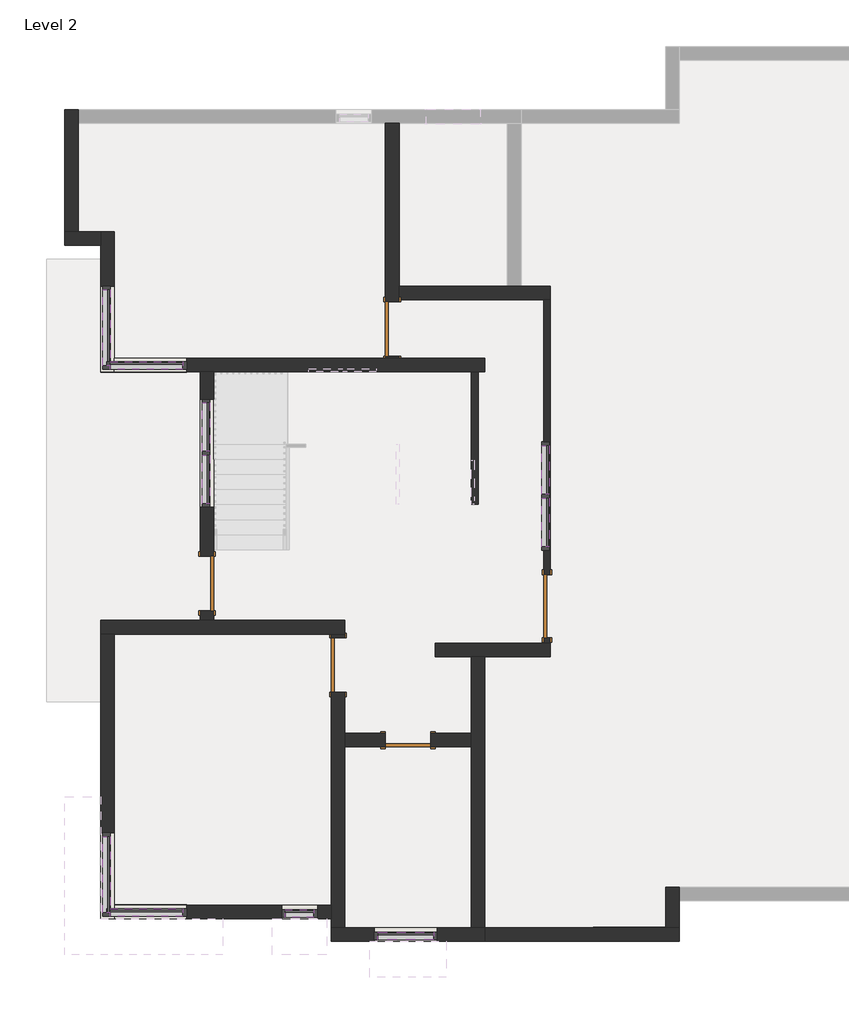
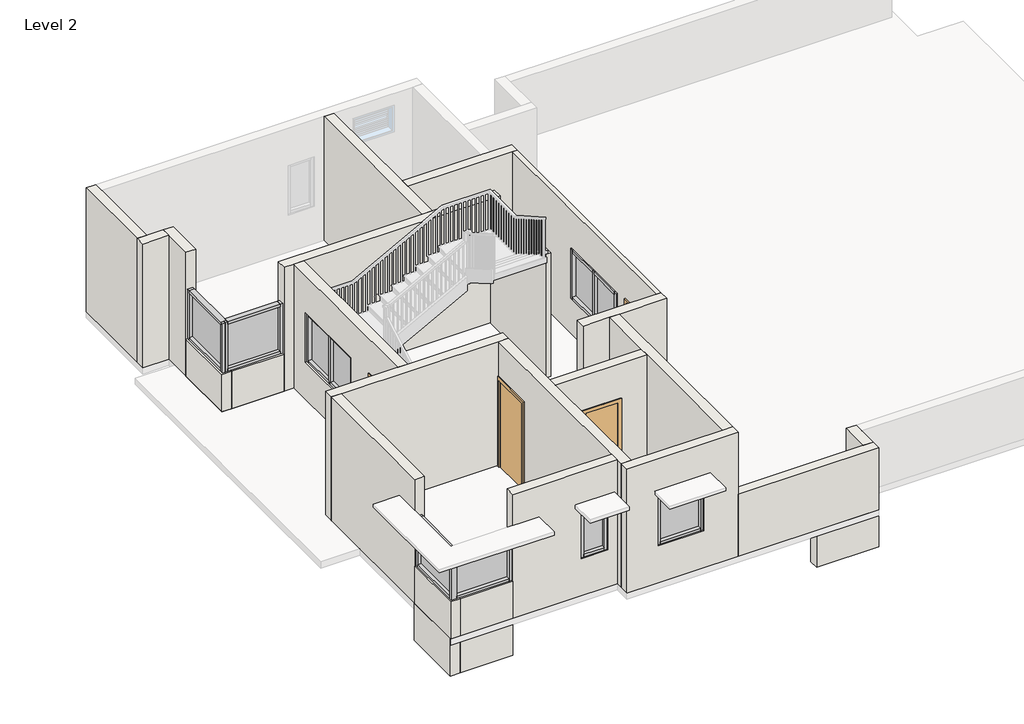
# One storey, part 1 of 5: 38 members, 29 walls, 10 plates, 5 doors.
"""IFC4 building model written with IfcOpenShell, lengths in millimetres."""

from ifc_helpers import new_model, si_unit, frame, origin, place, context, project, spatial, polyline, outline, extrude, faceted_brep, transform, mapped, element, save
from components import door_bb98abfd, single_flush_door_3_0ca8825f, single_flush_door_3_a90ba1ad, door_e6ebe4aa, member_75074519, member_05917e3b, member_5783932f, member_cba00588, member_c17f1be2, member_2b49869a, member_8d24a278, member_86d06fe4, member_e557a406, system_panel_glazed_87944ff9, system_panel_glazed_c8a97ecb, system_panel_glazed_1b15d1ca, system_panel_glazed_cc4caca5, system_panel_glazed_25f99c47, system_panel_glazed_1bcf12e0, system_panel_glazed_610bb4e0

model = new_model("IFC4")

# Units and contexts
model_context = context("Model", 3, world=origin())
ifc_project = project(units=[si_unit("LENGTHUNIT", "METRE", prefix="MILLI")], contexts=[model_context])

# Site, building, storey
site = spatial("IfcSite", under=ifc_project)
building = spatial("IfcBuilding", under=site)
storey = spatial("IfcBuildingStorey", under=building, Name="Level 2", Elevation=3048.0)

# Doors
placement = place(None, origin())
door_shape = door_bb98abfd(model_context)
element("IfcDoor", 1, ObjectType="Single-Flush : door 2'6\"", at=placement, inside=storey, context=model_context, shape_type="MappedRepresentation", body=[
    mapped(door_shape, transform((-37725.1146233, 9246.2080647, 3048.0), x_axis=(-1.0, 0.0, 0.0), y_axis=(0.0, -1.0, 0.0), z_axis=(0.0, 0.0, 1.0))),
])
single_flush_door_3_shape = single_flush_door_3_0ca8825f(model_context)
element("IfcDoor", 2, ObjectType="Single-Flush : door 3'", at=placement, inside=storey, context=model_context, shape_type="MappedRepresentation", body=[
    mapped(single_flush_door_3_shape, transform((-41116.0146233, 11887.8864709, 3048.0), x_axis=(0.0, -1.0, 0.0), y_axis=(1.0, 0.0, 0.0), z_axis=(0.0, 0.0, 1.0))),
])
element("IfcDoor", 3, ObjectType="Single-Flush : door 3'", at=placement, inside=storey, context=model_context, shape_type="MappedRepresentation", body=[
    mapped(single_flush_door_3_shape, transform((-38906.2146233, 10516.2864709, 3048.0), x_axis=(0.0, 1.0, 0.0), y_axis=(-1.0, 0.0, 0.0), z_axis=(0.0, 0.0, 1.0))),
])
single_flush_door_3_2_shape = single_flush_door_3_a90ba1ad(model_context)
element("IfcDoor", 4, ObjectType="Single-Flush : door 3'", at=placement, inside=storey, context=model_context, shape_type="MappedRepresentation", body=[
    mapped(single_flush_door_3_2_shape, transform((-37991.8146233, 16180.4864709, 3048.0), x_axis=(0.0, -1.0, 0.0), y_axis=(1.0, 0.0, 0.0), z_axis=(0.0, 0.0, 1.0))),
])
door_2_shape = door_e6ebe4aa(model_context)
element("IfcDoor", 5, ObjectType="Single-Flush : door 3'6\"", at=placement, inside=storey, context=model_context, shape_type="MappedRepresentation", body=[
    mapped(door_2_shape, transform((-35381.9646233, 11506.8864709, 3048.0), x_axis=(0.0, -1.0, 0.0), y_axis=(1.0, 0.0, 0.0), z_axis=(0.0, 0.0, 1.0))),
])

# Members
member_shape = member_75074519(model_context)
element("IfcMember", 6, ObjectType="Rectangular Mullion : 2.5\" x 5\" rectangular", at=placement, inside=storey, context=model_context, shape_type="MappedRepresentation", body=[
    mapped(member_shape, transform((-42808.6027511, 15501.0364709, 3962.4), x_axis=(0.0, -1.0, 0.0), y_axis=(-1.0, 0.0, 0.0), z_axis=(0.0, 0.0, -1.0))),
])
element("IfcMember", 7, ObjectType="Rectangular Mullion : 2.5\" x 5\" rectangular", at=placement, inside=storey, context=model_context, shape_type="MappedRepresentation", body=[
    mapped(member_shape, transform((-41458.9146233, 15564.5364709, 3962.4), x_axis=(1.0, 0.0, 0.0), y_axis=(0.0, -1.0, 0.0), z_axis=(0.0, 0.0, -1.0))),
])
element("IfcMember", 8, ObjectType="Rectangular Mullion : 2.5\" x 5\" rectangular", at=placement, inside=storey, context=model_context, shape_type="MappedRepresentation", body=[
    mapped(member_shape, transform((-42808.6027511, 6274.4882316, 3962.4), x_axis=(0.0, -1.0, 0.0), y_axis=(-1.0, 0.0, 0.0), z_axis=(0.0, 0.0, -1.0))),
])
element("IfcMember", 9, ObjectType="Rectangular Mullion : 2.5\" x 5\" rectangular", at=placement, inside=storey, context=model_context, shape_type="MappedRepresentation", body=[
    mapped(member_shape, transform((-41458.9146233, 6337.9882316, 3962.4), x_axis=(1.0, 0.0, 0.0), y_axis=(0.0, -1.0, 0.0), z_axis=(0.0, 0.0, -1.0))),
])
element("IfcMember", 10, ObjectType="Rectangular Mullion : 2.5\" x 5\" rectangular", at=placement, inside=storey, context=model_context, shape_type="MappedRepresentation", body=[
    mapped(member_shape, transform((-39249.1146233, 6325.2864709, 3962.4), x_axis=(1.0, 0.0, 0.0), y_axis=(0.0, -1.0, 0.0), z_axis=(0.0, 0.0, -1.0))),
])
element("IfcMember", 11, ObjectType="Rectangular Mullion : 2.5\" x 5\" rectangular", at=placement, inside=storey, context=model_context, shape_type="MappedRepresentation", body=[
    mapped(member_shape, transform((-37229.8146233, 5944.2080647, 3962.4), x_axis=(1.0, 0.0, 0.0), y_axis=(0.0, -1.0, 0.0), z_axis=(0.0, 0.0, -1.0))),
])
element("IfcMember", 12, ObjectType="Rectangular Mullion : 2.5\" x 5\" rectangular", at=placement, inside=storey, context=model_context, shape_type="MappedRepresentation", body=[
    mapped(member_shape, transform((-42808.6027511, 16904.3864709, 5181.6), x_axis=(0.0, 1.0, 0.0), y_axis=(-1.0, 0.0, 0.0), z_axis=(0.0, 0.0, 1.0))),
])
element("IfcMember", 13, ObjectType="Rectangular Mullion : 2.5\" x 5\" rectangular", at=placement, inside=storey, context=model_context, shape_type="MappedRepresentation", body=[
    mapped(member_shape, transform((-42808.6027511, 15564.5364709, 5181.6), x_axis=(-1.0, 0.0, 0.0), y_axis=(0.0, -1.0, 0.0), z_axis=(0.0, 0.0, 1.0))),
])
element("IfcMember", 14, ObjectType="Rectangular Mullion : 2.5\" x 5\" rectangular", at=placement, inside=storey, context=model_context, shape_type="MappedRepresentation", body=[
    mapped(member_shape, transform((-42808.6027511, 7684.1882316, 5181.6), x_axis=(0.0, 1.0, 0.0), y_axis=(-1.0, 0.0, 0.0), z_axis=(0.0, 0.0, 1.0))),
])
element("IfcMember", 15, ObjectType="Rectangular Mullion : 2.5\" x 5\" rectangular", at=placement, inside=storey, context=model_context, shape_type="MappedRepresentation", body=[
    mapped(member_shape, transform((-42808.6027511, 6337.9882316, 5181.6), x_axis=(-1.0, 0.0, 0.0), y_axis=(0.0, -1.0, 0.0), z_axis=(0.0, 0.0, 1.0))),
])
element("IfcMember", 16, ObjectType="Rectangular Mullion : 2.5\" x 5\" rectangular", at=placement, inside=storey, context=model_context, shape_type="MappedRepresentation", body=[
    mapped(member_shape, transform((-39858.7146233, 6325.2864709, 5181.6), x_axis=(-1.0, 0.0, 0.0), y_axis=(0.0, -1.0, 0.0), z_axis=(0.0, 0.0, 1.0))),
])
element("IfcMember", 17, ObjectType="Rectangular Mullion : 2.5\" x 5\" rectangular", at=placement, inside=storey, context=model_context, shape_type="MappedRepresentation", body=[
    mapped(member_shape, transform((-38296.6146233, 5944.2080647, 5181.6), x_axis=(-1.0, 0.0, 0.0), y_axis=(0.0, -1.0, 0.0), z_axis=(0.0, 0.0, 1.0))),
])
member_2_shape = member_05917e3b(model_context)
element("IfcMember", 18, ObjectType="Rectangular Mullion : 2.5\" x 5\" rectangular", at=placement, inside=storey, context=model_context, shape_type="MappedRepresentation", body=[
    mapped(member_2_shape, transform((-41522.4146233, 15564.5364709, 5181.6), x_axis=(0.0, 0.0, 1.0), y_axis=(0.0, -1.0, 0.0), z_axis=(1.0, 0.0, 0.0))),
])
element("IfcMember", 19, ObjectType="Rectangular Mullion : 2.5\" x 5\" rectangular", at=placement, inside=storey, context=model_context, shape_type="MappedRepresentation", body=[
    mapped(member_2_shape, transform((-41522.4146233, 6337.9882316, 5181.6), x_axis=(0.0, 0.0, 1.0), y_axis=(0.0, -1.0, 0.0), z_axis=(1.0, 0.0, 0.0))),
])
element("IfcMember", 20, ObjectType="Rectangular Mullion : 2.5\" x 5\" rectangular", at=placement, inside=storey, context=model_context, shape_type="MappedRepresentation", body=[
    mapped(member_2_shape, transform((-42745.1027511, 15564.5364709, 3962.4), x_axis=(0.0, 0.0, -1.0), y_axis=(0.0, -1.0, 0.0), z_axis=(-1.0, 0.0, 0.0))),
])
element("IfcMember", 21, ObjectType="Rectangular Mullion : 2.5\" x 5\" rectangular", at=placement, inside=storey, context=model_context, shape_type="MappedRepresentation", body=[
    mapped(member_2_shape, transform((-42745.1027511, 6337.9882316, 3962.4), x_axis=(0.0, 0.0, -1.0), y_axis=(0.0, -1.0, 0.0), z_axis=(-1.0, 0.0, 0.0))),
])
member_3_shape = member_5783932f(model_context)
element("IfcMember", 22, ObjectType="Rectangular Mullion : 2.5\" x 5\" rectangular", at=placement, inside=storey, context=model_context, shape_type="MappedRepresentation", body=[
    mapped(member_3_shape, transform((-42808.6027511, 6337.9882316, 5181.6), x_axis=(0.0, 0.0, 1.0), y_axis=(-1.0, 0.0, 0.0), z_axis=(0.0, -1.0, 0.0))),
])
element("IfcMember", 23, ObjectType="Rectangular Mullion : 2.5\" x 5\" rectangular", at=placement, inside=storey, context=model_context, shape_type="MappedRepresentation", body=[
    mapped(member_3_shape, transform((-42808.6027511, 7620.6882316, 3962.4), x_axis=(0.0, 0.0, -1.0), y_axis=(-1.0, 0.0, 0.0), z_axis=(0.0, 1.0, 0.0))),
])
member_4_shape = member_cba00588(model_context)
element("IfcMember", 24, ObjectType="Rectangular Mullion : 2.5\" x 5\" rectangular", at=placement, inside=storey, context=model_context, shape_type="MappedRepresentation", body=[
    mapped(member_4_shape, transform((-42808.6027511, 15564.5364709, 5181.6), x_axis=(0.0, 0.0, 1.0), y_axis=(-1.0, 0.0, 0.0), z_axis=(0.0, -1.0, 0.0))),
])
element("IfcMember", 25, ObjectType="Rectangular Mullion : 2.5\" x 5\" rectangular", at=placement, inside=storey, context=model_context, shape_type="MappedRepresentation", body=[
    mapped(member_4_shape, transform((-42808.6027511, 16840.8864709, 3962.4), x_axis=(0.0, 0.0, -1.0), y_axis=(-1.0, 0.0, 0.0), z_axis=(0.0, 1.0, 0.0))),
])
member_5_shape = member_c17f1be2(model_context)
element("IfcMember", 26, ObjectType="Rectangular Mullion : 2.5\" x 5\" rectangular", at=placement, inside=storey, context=model_context, shape_type="MappedRepresentation", body=[
    mapped(member_5_shape, transform((-41132.1878805, 14935.8864709, 5181.6), x_axis=(0.0, 0.0, 1.0), y_axis=(1.0, 0.0, 0.0), z_axis=(0.0, 1.0, 0.0))),
])
element("IfcMember", 27, ObjectType="Rectangular Mullion : 2.5\" x 5\" rectangular", at=placement, inside=storey, context=model_context, shape_type="MappedRepresentation", body=[
    mapped(member_5_shape, transform((-41132.1878805, 14053.2364709, 5181.6), x_axis=(0.0, 0.0, 1.0), y_axis=(1.0, 0.0, 0.0), z_axis=(0.0, 1.0, 0.0))),
])
element("IfcMember", 28, ObjectType="Rectangular Mullion : 2.5\" x 5\" rectangular", at=placement, inside=storey, context=model_context, shape_type="MappedRepresentation", body=[
    mapped(member_5_shape, transform((-41132.1878805, 13234.0864709, 3962.4), x_axis=(0.0, 0.0, -1.0), y_axis=(1.0, 0.0, 0.0), z_axis=(0.0, -1.0, 0.0))),
])
element("IfcMember", 29, ObjectType="Rectangular Mullion : 2.5\" x 5\" rectangular", at=placement, inside=storey, context=model_context, shape_type="MappedRepresentation", body=[
    mapped(member_5_shape, transform((-41132.1878805, 14116.7364709, 3962.4), x_axis=(0.0, 0.0, -1.0), y_axis=(1.0, 0.0, 0.0), z_axis=(0.0, -1.0, 0.0))),
])
member_6_shape = member_2b49869a(model_context)
element("IfcMember", 30, ObjectType="Rectangular Mullion : 2.5\" x 5\" rectangular", at=placement, inside=storey, context=model_context, shape_type="MappedRepresentation", body=[
    mapped(member_6_shape, transform((-41132.1878805, 14084.9864709, 3962.4), x_axis=(0.0, 1.0, 0.0), y_axis=(1.0, 0.0, 0.0), z_axis=(0.0, 0.0, -1.0))),
])
element("IfcMember", 31, ObjectType="Rectangular Mullion : 2.5\" x 5\" rectangular", at=placement, inside=storey, context=model_context, shape_type="MappedRepresentation", body=[
    mapped(member_6_shape, transform((-35404.4407526, 13360.7894527, 3962.4), x_axis=(0.0, 1.0, 0.0), y_axis=(1.0, 0.0, 0.0), z_axis=(0.0, 0.0, -1.0))),
])
element("IfcMember", 32, ObjectType="Rectangular Mullion : 2.5\" x 5\" rectangular", at=placement, inside=storey, context=model_context, shape_type="MappedRepresentation", body=[
    mapped(member_shape, transform((-41132.1878805, 14999.3864709, 3962.4), x_axis=(0.0, 1.0, 0.0), y_axis=(1.0, 0.0, 0.0), z_axis=(0.0, 0.0, -1.0))),
])
element("IfcMember", 33, ObjectType="Rectangular Mullion : 2.5\" x 5\" rectangular", at=placement, inside=storey, context=model_context, shape_type="MappedRepresentation", body=[
    mapped(member_shape, transform((-35404.4407526, 14274.8924345, 3962.4), x_axis=(0.0, 1.0, 0.0), y_axis=(1.0, 0.0, 0.0), z_axis=(0.0, 0.0, -1.0))),
])
element("IfcMember", 34, ObjectType="Rectangular Mullion : 2.5\" x 5\" rectangular", at=placement, inside=storey, context=model_context, shape_type="MappedRepresentation", body=[
    mapped(member_shape, transform((-41132.1878805, 13170.5864709, 5181.6), x_axis=(0.0, -1.0, 0.0), y_axis=(1.0, 0.0, 0.0), z_axis=(0.0, 0.0, 1.0))),
])
element("IfcMember", 35, ObjectType="Rectangular Mullion : 2.5\" x 5\" rectangular", at=placement, inside=storey, context=model_context, shape_type="MappedRepresentation", body=[
    mapped(member_shape, transform((-35404.4407526, 12446.6864709, 5181.6), x_axis=(0.0, -1.0, 0.0), y_axis=(1.0, 0.0, 0.0), z_axis=(0.0, 0.0, 1.0))),
])
member_7_shape = member_8d24a278(model_context)
element("IfcMember", 36, ObjectType="Rectangular Mullion : 2.5\" x 5\" rectangular", at=placement, inside=storey, context=model_context, shape_type="MappedRepresentation", body=[
    mapped(member_7_shape, transform((-35404.4407526, 14211.3924345, 5181.6), x_axis=(0.0, 0.0, 1.0), y_axis=(1.0, 0.0, 0.0), z_axis=(0.0, 1.0, 0.0))),
])
element("IfcMember", 37, ObjectType="Rectangular Mullion : 2.5\" x 5\" rectangular", at=placement, inside=storey, context=model_context, shape_type="MappedRepresentation", body=[
    mapped(member_7_shape, transform((-35404.4407526, 13329.0394527, 5181.6), x_axis=(0.0, 0.0, 1.0), y_axis=(1.0, 0.0, 0.0), z_axis=(0.0, 1.0, 0.0))),
])
element("IfcMember", 38, ObjectType="Rectangular Mullion : 2.5\" x 5\" rectangular", at=placement, inside=storey, context=model_context, shape_type="MappedRepresentation", body=[
    mapped(member_7_shape, transform((-35404.4407526, 12510.1864709, 3962.4), x_axis=(0.0, 0.0, -1.0), y_axis=(1.0, 0.0, 0.0), z_axis=(0.0, -1.0, 0.0))),
])
element("IfcMember", 39, ObjectType="Rectangular Mullion : 2.5\" x 5\" rectangular", at=placement, inside=storey, context=model_context, shape_type="MappedRepresentation", body=[
    mapped(member_7_shape, transform((-35404.4407526, 13392.5394527, 3962.4), x_axis=(0.0, 0.0, -1.0), y_axis=(1.0, 0.0, 0.0), z_axis=(0.0, -1.0, 0.0))),
])
member_8_shape = member_86d06fe4(model_context)
element("IfcMember", 40, ObjectType="Rectangular Mullion : 2.5\" x 5\" rectangular", at=placement, inside=storey, context=model_context, shape_type="MappedRepresentation", body=[
    mapped(member_8_shape, transform((-39312.6146233, 6325.2864709, 5181.6), x_axis=(0.0, 0.0, 1.0), y_axis=(0.0, -1.0, 0.0), z_axis=(1.0, 0.0, 0.0))),
])
element("IfcMember", 41, ObjectType="Rectangular Mullion : 2.5\" x 5\" rectangular", at=placement, inside=storey, context=model_context, shape_type="MappedRepresentation", body=[
    mapped(member_8_shape, transform((-39795.2146233, 6325.2864709, 3962.4), x_axis=(0.0, 0.0, -1.0), y_axis=(0.0, -1.0, 0.0), z_axis=(-1.0, 0.0, 0.0))),
])
member_9_shape = member_e557a406(model_context)
element("IfcMember", 42, ObjectType="Rectangular Mullion : 2.5\" x 5\" rectangular", at=placement, inside=storey, context=model_context, shape_type="MappedRepresentation", body=[
    mapped(member_9_shape, transform((-37293.3146233, 5944.2080647, 5181.6), x_axis=(0.0, 0.0, 1.0), y_axis=(0.0, -1.0, 0.0), z_axis=(1.0, 0.0, 0.0))),
])
element("IfcMember", 43, ObjectType="Rectangular Mullion : 2.5\" x 5\" rectangular", at=placement, inside=storey, context=model_context, shape_type="MappedRepresentation", body=[
    mapped(member_9_shape, transform((-38233.1146233, 5944.2080647, 3962.4), x_axis=(0.0, 0.0, -1.0), y_axis=(0.0, -1.0, 0.0), z_axis=(-1.0, 0.0, 0.0))),
])

# Plates
system_panel_glazed_shape = system_panel_glazed_87944ff9(model_context)
element("IfcPlate", 44, ObjectType="System Panel : Glazed", at=placement, inside=storey, context=model_context, shape_type="MappedRepresentation", body=[
    mapped(system_panel_glazed_shape, transform((-42808.6027511, 6979.3382316, 4025.9), x_axis=(0.0, -1.0, 0.0), y_axis=(1.0, 0.0, 0.0), z_axis=(0.0, 0.0, 1.0))),
])
system_panel_glazed_2_shape = system_panel_glazed_c8a97ecb(model_context)
element("IfcPlate", 45, ObjectType="System Panel : Glazed", at=placement, inside=storey, context=model_context, shape_type="MappedRepresentation", body=[
    mapped(system_panel_glazed_2_shape, transform((-42133.7586872, 15564.5364709, 4025.9), x_axis=(1.0, 0.0, 0.0), y_axis=(0.0, 1.0, 0.0), z_axis=(0.0, 0.0, 1.0))),
])
element("IfcPlate", 46, ObjectType="System Panel : Glazed", at=placement, inside=storey, context=model_context, shape_type="MappedRepresentation", body=[
    mapped(system_panel_glazed_2_shape, transform((-42133.7586872, 6337.9882316, 4025.9), x_axis=(1.0, 0.0, 0.0), y_axis=(0.0, 1.0, 0.0), z_axis=(0.0, 0.0, 1.0))),
])
system_panel_glazed_3_shape = system_panel_glazed_1b15d1ca(model_context)
element("IfcPlate", 47, ObjectType="System Panel : Glazed", at=placement, inside=storey, context=model_context, shape_type="MappedRepresentation", body=[
    mapped(system_panel_glazed_3_shape, transform((-42808.6027511, 16202.7114709, 4025.9), x_axis=(0.0, -1.0, 0.0), y_axis=(1.0, 0.0, 0.0), z_axis=(0.0, 0.0, 1.0))),
])
system_panel_glazed_4_shape = system_panel_glazed_cc4caca5(model_context)
element("IfcPlate", 48, ObjectType="System Panel : Glazed", at=placement, inside=storey, context=model_context, shape_type="MappedRepresentation", body=[
    mapped(system_panel_glazed_4_shape, transform((-41132.1878805, 13643.6614709, 4025.9), x_axis=(0.0, 1.0, 0.0), y_axis=(-1.0, 0.0, 0.0), z_axis=(0.0, 0.0, 1.0))),
])
element("IfcPlate", 49, ObjectType="System Panel : Glazed", at=placement, inside=storey, context=model_context, shape_type="MappedRepresentation", body=[
    mapped(system_panel_glazed_4_shape, transform((-41132.1878805, 14526.3114709, 4025.9), x_axis=(0.0, 1.0, 0.0), y_axis=(-1.0, 0.0, 0.0), z_axis=(0.0, 0.0, 1.0))),
])
system_panel_glazed_5_shape = system_panel_glazed_25f99c47(model_context)
element("IfcPlate", 50, ObjectType="System Panel : Glazed", at=placement, inside=storey, context=model_context, shape_type="MappedRepresentation", body=[
    mapped(system_panel_glazed_5_shape, transform((-35404.4407526, 12919.6129618, 4025.9), x_axis=(0.0, 1.0, 0.0), y_axis=(-1.0, 0.0, 0.0), z_axis=(0.0, 0.0, 1.0))),
])
element("IfcPlate", 51, ObjectType="System Panel : Glazed", at=placement, inside=storey, context=model_context, shape_type="MappedRepresentation", body=[
    mapped(system_panel_glazed_5_shape, transform((-35404.4407526, 13801.9659436, 4025.9), x_axis=(0.0, 1.0, 0.0), y_axis=(-1.0, 0.0, 0.0), z_axis=(0.0, 0.0, 1.0))),
])
system_panel_glazed_6_shape = system_panel_glazed_1bcf12e0(model_context)
element("IfcPlate", 52, ObjectType="System Panel : Glazed", at=placement, inside=storey, context=model_context, shape_type="MappedRepresentation", body=[
    mapped(system_panel_glazed_6_shape, transform((-39553.9146233, 6325.2864709, 4025.9), x_axis=(1.0, 0.0, 0.0), y_axis=(0.0, 1.0, 0.0), z_axis=(0.0, 0.0, 1.0))),
])
system_panel_glazed_7_shape = system_panel_glazed_610bb4e0(model_context)
element("IfcPlate", 53, ObjectType="System Panel : Glazed", at=placement, inside=storey, context=model_context, shape_type="MappedRepresentation", body=[
    mapped(system_panel_glazed_7_shape, transform((-37763.2146233, 5944.2080647, 4025.9), x_axis=(1.0, 0.0, 0.0), y_axis=(0.0, 1.0, 0.0), z_axis=(0.0, 0.0, 1.0))),
])

# Walls
element("IfcWall", 54, at=placement, inside=storey, context=model_context, shape_type="Brep", body=[
    faceted_brep([(-36429.7146233, 5855.3080647, 3048.0), (-33153.1146233, 5855.3080647, 3048.0), (-33153.1146233, 5855.3080647, 4572.0), (-36429.7146233, 5855.3080647, 4572.0), (-36429.7146233, 6083.9080647, 3048.0), (-36429.7146233, 6083.9080647, 4572.0), (-33381.7146233, 6083.9080647, 4572.0), (-33153.1146233, 6083.9080647, 4572.0), (-33153.1146233, 6083.9080647, 3048.0), (-33381.7146233, 6083.9080647, 3048.0)], [[[0, 1, 2, 3]], [[4, 5, 6, 7, 8, 9]], [[1, 0, 4, 9, 8]], [[3, 2, 7, 6, 5]], [[2, 1, 8, 7]], [[0, 3, 5, 4]]]),
])
element("IfcWall", 55, at=placement, inside=storey, context=model_context, shape_type="Brep", body=[
    faceted_brep([(-33153.1146233, 6083.9080647, 3048.0), (-33153.1146233, 6541.1864709, 3048.0), (-33153.1146233, 6769.7864709, 3048.0), (-33153.1146233, 6769.7864709, 4572.0), (-33153.1146233, 6541.1864709, 4572.0), (-33153.1146233, 6083.9080647, 4572.0), (-33381.7146233, 6083.9080647, 3048.0), (-33381.7146233, 6083.9080647, 4572.0), (-33381.7146233, 6769.7864709, 4572.0), (-33381.7146233, 6769.7864709, 3048.0)], [[[0, 1, 2, 3, 4, 5]], [[6, 7, 8, 9]], [[2, 1, 0, 6, 9]], [[5, 4, 3, 8, 7]], [[0, 5, 7, 6]], [[3, 2, 9, 8]]]),
])
element("IfcWall", 56, ObjectType="Generic - 5\"", at=placement, inside=storey, context=model_context, shape_type="SweptSolid", body=[
    extrude(outline(polyline([(-36658.3146233, 13221.3864709), (-36658.3146233, 15456.5864709), (-36544.0146233, 15456.5864709), (-36544.0146233, 13221.3864709), (-36658.3146233, 13221.3864709)])), frame((0.0, 0.0, 3048.0), z_axis=(0.0, 0.0, 1.0), x_axis=(1.0, 0.0, 0.0)), (0.0, 0.0, 1.0), 3048.0),
])
element("IfcWall", 57, ObjectType="WALL 9\"", at=placement, inside=storey, context=model_context, shape_type="Brep", body=[
    faceted_brep([(-42678.1146233, 16904.3864709, 6096.0), (-42678.1146233, 16904.3864709, 5181.6), (-42678.1146233, 16904.3864709, 3962.4), (-42678.1146233, 16904.3864709, 3048.0), (-42678.1146233, 17818.7864709, 3048.0), (-42678.1146233, 17818.7864709, 6096.0), (-42906.7146233, 16904.3864709, 3048.0), (-42906.7146233, 16904.3864709, 3962.4), (-42906.7146233, 16904.3864709, 5181.6), (-42906.7146233, 16904.3864709, 6096.0), (-42906.7146233, 17590.1864709, 6096.0), (-42906.7146233, 17818.7864709, 6096.0), (-42906.7146233, 17818.7864709, 3048.0), (-42906.7146233, 17590.1864709, 3048.0)], [[[0, 1, 2, 3, 4, 5]], [[6, 7, 8, 9, 10, 11, 12, 13]], [[4, 3, 6, 13, 12]], [[0, 9, 8, 7, 6, 3, 2, 1]], [[0, 5, 11, 10, 9]], [[5, 4, 12, 11]]]),
])
element("IfcWall", 58, ObjectType="WALL 9\"", at=placement, inside=storey, context=model_context, shape_type="Brep", body=[
    faceted_brep([(-42906.7146233, 17818.7864709, 3048.0), (-43287.7146233, 17818.7864709, 3048.0), (-43516.3146233, 17818.7864709, 3048.0), (-43516.3146233, 17818.7864709, 6096.0), (-43287.7146233, 17818.7864709, 6096.0), (-42906.7146233, 17818.7864709, 6096.0), (-42906.7146233, 17590.1864709, 3048.0), (-42906.7146233, 17590.1864709, 6096.0), (-43516.3146233, 17590.1864709, 6096.0), (-43516.3146233, 17590.1864709, 3048.0)], [[[0, 1, 2, 3, 4, 5]], [[6, 7, 8, 9]], [[2, 1, 0, 6, 9]], [[5, 4, 3, 8, 7]], [[3, 2, 9, 8]], [[0, 5, 7, 6]]]),
])
element("IfcWall", 59, ObjectType="WALL 9\"", at=placement, inside=storey, context=model_context, shape_type="Brep", body=[
    faceted_brep([(-43287.7146233, 17818.7864709, 3048.0), (-43287.7146233, 19647.5864709, 3048.0), (-43287.7146233, 19876.1864709, 3048.0), (-43287.7146233, 19876.1864709, 6096.0), (-43287.7146233, 19647.5864709, 6096.0), (-43287.7146233, 17818.7864709, 6096.0), (-43516.3146233, 17818.7864709, 3048.0), (-43516.3146233, 17818.7864709, 6096.0), (-43516.3146233, 19876.1864709, 6096.0), (-43516.3146233, 19876.1864709, 3048.0)], [[[0, 1, 2, 3, 4, 5]], [[6, 7, 8, 9]], [[2, 1, 0, 6, 9]], [[5, 4, 3, 8, 7]], [[3, 2, 9, 8]], [[0, 5, 7, 6]]]),
])
element("IfcWall", 60, ObjectType="WALL 9\"", at=placement, inside=storey, context=model_context, shape_type="Brep", body=[
    faceted_brep([(-41458.9146233, 15456.5864709, 6096.0), (-41458.9146233, 15456.5864709, 5181.6), (-41458.9146233, 15456.5864709, 3962.4), (-41458.9146233, 15456.5864709, 3048.0), (-41230.3146233, 15456.5864709, 3048.0), (-41001.7146233, 15456.5864709, 3048.0), (-36658.3146233, 15456.5864709, 3048.0), (-36544.0146233, 15456.5864709, 3048.0), (-36429.7146233, 15456.5864709, 3048.0), (-36429.7146233, 15456.5864709, 6096.0), (-36544.0146233, 15456.5864709, 6096.0), (-36658.3146233, 15456.5864709, 6096.0), (-41001.7146233, 15456.5864709, 6096.0), (-41230.3146233, 15456.5864709, 6096.0), (-41458.9146233, 15685.1864709, 3048.0), (-41458.9146233, 15685.1864709, 3962.4), (-41458.9146233, 15685.1864709, 5181.6), (-41458.9146233, 15685.1864709, 6096.0), (-38106.1146233, 15685.1864709, 6096.0), (-37877.5146233, 15685.1864709, 6096.0), (-36429.7146233, 15685.1864709, 6096.0), (-36429.7146233, 15685.1864709, 3048.0), (-37877.5146233, 15685.1864709, 3048.0), (-38106.1146233, 15685.1864709, 3048.0)], [[[0, 1, 2, 3, 4, 5, 6, 7, 8, 9, 10, 11, 12, 13]], [[14, 15, 16, 17, 18, 19, 20, 21, 22, 23]], [[8, 7, 6, 5, 4, 3, 14, 23, 22, 21]], [[9, 8, 21, 20]], [[0, 17, 16, 15, 14, 3, 2, 1]], [[0, 13, 12, 11, 10, 9, 20, 19, 18, 17]]]),
])
element("IfcWall", 61, ObjectType="WALL 9\"", at=placement, inside=storey, context=model_context, shape_type="Brep", body=[
    faceted_brep([(-38106.1146233, 15723.2864709, 5181.6), (-38106.1146233, 15723.2864709, 3048.0), (-38106.1146233, 15685.1864709, 3048.0), (-38106.1146233, 15685.1864709, 6096.0), (-38106.1146233, 19647.5864709, 6096.0), (-38106.1146233, 19647.5864709, 3048.0), (-38106.1146233, 16637.6864709, 3048.0), (-38106.1146233, 16637.6864709, 5181.6), (-37877.5146233, 15685.1864709, 3048.0), (-37877.5146233, 15723.2864709, 3048.0), (-37877.5146233, 15723.2864709, 5181.6), (-37877.5146233, 16637.6864709, 5181.6), (-37877.5146233, 16637.6864709, 3048.0), (-37877.5146233, 16675.7864709, 3048.0), (-37877.5146233, 16904.3864709, 3048.0), (-37877.5146233, 19647.5864709, 3048.0), (-37877.5146233, 19647.5864709, 6096.0), (-37877.5146233, 16904.3864709, 6096.0), (-37877.5146233, 16675.7864709, 6096.0), (-37877.5146233, 15685.1864709, 6096.0)], [[[0, 1, 2, 3, 4, 5, 6, 7]], [[8, 9, 10, 11, 12, 13, 14, 15, 16, 17, 18, 19]], [[6, 5, 15, 14, 13, 12]], [[2, 1, 9, 8]], [[5, 4, 16, 15]], [[3, 2, 8, 19]], [[10, 9, 1, 0]], [[11, 10, 0, 7]], [[12, 11, 7, 6]], [[4, 3, 19, 18, 17, 16]]]),
])
element("IfcWall", 62, ObjectType="WALL 9\"", at=placement, inside=storey, context=model_context, shape_type="Brep", body=[
    faceted_brep([(-37877.5146233, 16675.7864709, 3048.0), (-35439.1146233, 16675.7864709, 3048.0), (-35324.8146233, 16675.7864709, 3048.0), (-35324.8146233, 16675.7864709, 6096.0), (-35439.1146233, 16675.7864709, 6096.0), (-37877.5146233, 16675.7864709, 6096.0), (-37877.5146233, 16904.3864709, 3048.0), (-37877.5146233, 16904.3864709, 6096.0), (-36048.7146233, 16904.3864709, 6096.0), (-35820.1146233, 16904.3864709, 6096.0), (-35324.8146233, 16904.3864709, 6096.0), (-35324.8146233, 16904.3864709, 3048.0), (-35820.1146233, 16904.3864709, 3048.0), (-36048.7146233, 16904.3864709, 3048.0)], [[[0, 1, 2, 3, 4, 5]], [[6, 7, 8, 9, 10, 11, 12, 13]], [[2, 1, 0, 6, 13, 12, 11]], [[0, 5, 7, 6]], [[5, 4, 3, 10, 9, 8, 7]], [[3, 2, 11, 10]]]),
])
element("IfcWall", 63, ObjectType="WALL 9\"", at=placement, inside=storey, context=model_context, shape_type="Brep", body=[
    faceted_brep([(-41230.3146233, 15456.5864709, 6096.0), (-41230.3146233, 15456.5864709, 3048.0), (-41230.3146233, 12345.0864709, 3048.0), (-41230.3146233, 12345.0864709, 5181.6), (-41230.3146233, 11430.6864709, 5181.6), (-41230.3146233, 11430.6864709, 3048.0), (-41230.3146233, 11265.5864709, 3048.0), (-41230.3146233, 11265.5864709, 6096.0), (-41230.3146233, 13170.5864709, 5181.6), (-41230.3146233, 13170.5864709, 3962.4), (-41230.3146233, 14999.3864709, 3962.4), (-41230.3146233, 14999.3864709, 5181.6), (-41001.7146233, 15456.5864709, 3048.0), (-41001.7146233, 15456.5864709, 6096.0), (-41001.7146233, 12459.3864709, 6096.0), (-41001.7146233, 11265.5864709, 6096.0), (-41001.7146233, 11265.5864709, 3048.0), (-41001.7146233, 11430.6864709, 3048.0), (-41001.7146233, 11430.6864709, 5181.6), (-41001.7146233, 12345.0864709, 5181.6), (-41001.7146233, 12345.0864709, 3048.0), (-41001.7146233, 13170.5864709, 3962.4), (-41001.7146233, 13170.5864709, 5181.6), (-41001.7146233, 14999.3864709, 5181.6), (-41001.7146233, 14999.3864709, 3962.4)], [[[0, 1, 2, 3, 4, 5, 6, 7], [8, 9, 10, 11]], [[12, 13, 14, 15, 16, 17, 18, 19, 20], [21, 22, 23, 24]], [[1, 12, 20, 2]], [[16, 6, 5, 17]], [[1, 0, 13, 12]], [[7, 6, 16, 15]], [[21, 9, 8, 22]], [[22, 8, 11, 23]], [[23, 11, 10, 24]], [[9, 21, 24, 10]], [[18, 17, 5, 4]], [[19, 18, 4, 3]], [[20, 19, 3, 2]], [[13, 0, 7, 15, 14]]]),
])
element("IfcWall", 64, ObjectType="WALL 9\"", at=placement, inside=storey, context=model_context, shape_type="Brep", body=[
    faceted_brep([(-42906.7146233, 11036.9864709, 3048.0), (-42678.1146233, 11036.9864709, 3048.0), (-39020.5146233, 11036.9864709, 3048.0), (-38791.9146233, 11036.9864709, 3048.0), (-38791.9146233, 11036.9864709, 6096.0), (-39020.5146233, 11036.9864709, 6096.0), (-42678.1146233, 11036.9864709, 6096.0), (-42906.7146233, 11036.9864709, 6096.0), (-42906.7146233, 11265.5864709, 3048.0), (-42906.7146233, 11265.5864709, 6096.0), (-41230.3146233, 11265.5864709, 6096.0), (-41001.7146233, 11265.5864709, 6096.0), (-38791.9146233, 11265.5864709, 6096.0), (-38791.9146233, 11265.5864709, 3048.0), (-41001.7146233, 11265.5864709, 3048.0), (-41230.3146233, 11265.5864709, 3048.0)], [[[0, 1, 2, 3, 4, 5, 6, 7]], [[8, 9, 10, 11, 12, 13, 14, 15]], [[3, 2, 1, 0, 8, 15, 14, 13]], [[4, 3, 13, 12]], [[7, 6, 5, 4, 12, 11, 10, 9]], [[0, 7, 9, 8]]]),
])
element("IfcWall", 65, ObjectType="WALL 9\"", at=placement, inside=storey, context=model_context, shape_type="Brep", body=[
    faceted_brep([(-42906.7146233, 11036.9864709, 3048.0), (-42906.7146233, 7684.1882316, 3048.0), (-42906.7146233, 7684.1882316, 3962.4), (-42906.7146233, 7684.1882316, 5181.6), (-42906.7146233, 7684.1882316, 6096.0), (-42906.7146233, 11036.9864709, 6096.0), (-42678.1146233, 11036.9864709, 3048.0), (-42678.1146233, 11036.9864709, 6096.0), (-42678.1146233, 7684.1882316, 6096.0), (-42678.1146233, 7684.1882316, 5181.6), (-42678.1146233, 7684.1882316, 3962.4), (-42678.1146233, 7684.1882316, 3048.0)], [[[0, 1, 2, 3, 4, 5]], [[6, 7, 8, 9, 10, 11]], [[1, 0, 6, 11]], [[1, 11, 10, 9, 8, 4, 3, 2]], [[5, 4, 8, 7]], [[0, 5, 7, 6]]]),
])
element("IfcWall", 66, ObjectType="WALL 9\"", at=placement, inside=storey, context=model_context, shape_type="Brep", body=[
    faceted_brep([(-41458.9146233, 6236.3864709, 3048.0), (-39020.5146233, 6236.3864709, 3048.0), (-39020.5146233, 6236.3864709, 6096.0), (-41458.9146233, 6236.3864709, 6096.0), (-41458.9146233, 6236.3864709, 5181.6), (-41458.9146233, 6236.3864709, 3962.4), (-39858.7146233, 6236.3864709, 3962.4), (-39858.7146233, 6236.3864709, 5181.6), (-39249.1146233, 6236.3864709, 5181.6), (-39249.1146233, 6236.3864709, 3962.4), (-39020.5146233, 6464.9864709, 3048.0), (-41458.9146233, 6464.9864709, 3048.0), (-41458.9146233, 6464.9864709, 3962.4), (-41458.9146233, 6464.9864709, 5181.6), (-41458.9146233, 6464.9864709, 6096.0), (-39020.5146233, 6464.9864709, 6096.0), (-39858.7146233, 6464.9864709, 5181.6), (-39858.7146233, 6464.9864709, 3962.4), (-39249.1146233, 6464.9864709, 3962.4), (-39249.1146233, 6464.9864709, 5181.6)], [[[0, 1, 2, 3, 4, 5], [6, 7, 8, 9]], [[10, 11, 12, 13, 14, 15], [16, 17, 18, 19]], [[1, 0, 11, 10]], [[2, 1, 10, 15]], [[11, 0, 5, 4, 3, 14, 13, 12]], [[6, 17, 16, 7]], [[7, 16, 19, 8]], [[8, 19, 18, 9]], [[17, 6, 9, 18]], [[3, 2, 15, 14]]]),
])
element("IfcWall", 67, ObjectType="WALL 9\"", at=placement, inside=storey, context=model_context, shape_type="Brep", body=[
    faceted_brep([(-39020.5146233, 5855.3080647, 3048.0), (-36429.7146233, 5855.3080647, 3048.0), (-36429.7146233, 5855.3080647, 4572.0), (-36429.7146233, 5855.3080647, 6096.0), (-39020.5146233, 5855.3080647, 6096.0), (-38296.6146233, 5855.3080647, 3962.4), (-38296.6146233, 5855.3080647, 5181.6), (-37229.8146233, 5855.3080647, 5181.6), (-37229.8146233, 5855.3080647, 3962.4), (-36429.7146233, 6083.9080647, 3048.0), (-36658.3146233, 6083.9080647, 3048.0), (-38791.9146233, 6083.9080647, 3048.0), (-39020.5146233, 6083.9080647, 3048.0), (-39020.5146233, 6083.9080647, 6096.0), (-38791.9146233, 6083.9080647, 6096.0), (-36658.3146233, 6083.9080647, 6096.0), (-36429.7146233, 6083.9080647, 6096.0), (-36429.7146233, 6083.9080647, 4572.0), (-38296.6146233, 6083.9080647, 5181.6), (-38296.6146233, 6083.9080647, 3962.4), (-37229.8146233, 6083.9080647, 3962.4), (-37229.8146233, 6083.9080647, 5181.6)], [[[0, 1, 2, 3, 4], [5, 6, 7, 8]], [[9, 10, 11, 12, 13, 14, 15, 16, 17], [18, 19, 20, 21]], [[1, 0, 12, 11, 10, 9]], [[5, 19, 18, 6]], [[6, 18, 21, 7]], [[7, 21, 20, 8]], [[19, 5, 8, 20]], [[4, 3, 16, 15, 14, 13]], [[0, 4, 13, 12]], [[1, 9, 17, 16, 3, 2]]]),
])
element("IfcWall", 68, ObjectType="WALL 9\"", at=placement, inside=storey, context=model_context, shape_type="Brep", body=[
    faceted_brep([(-36429.7146233, 6083.9080647, 6096.0), (-36429.7146233, 6083.9080647, 3048.0), (-36429.7146233, 10655.9864709, 3048.0), (-36429.7146233, 10655.9864709, 6096.0), (-36658.3146233, 6083.9080647, 3048.0), (-36658.3146233, 6083.9080647, 6096.0), (-36658.3146233, 9131.9080647, 6096.0), (-36658.3146233, 9360.5080647, 6096.0), (-36658.3146233, 10655.9864709, 6096.0), (-36658.3146233, 10655.9864709, 3048.0), (-36658.3146233, 9360.5080647, 3048.0), (-36658.3146233, 9131.9080647, 3048.0)], [[[0, 1, 2, 3]], [[4, 5, 6, 7, 8, 9, 10, 11]], [[2, 1, 4, 11, 10, 9]], [[3, 2, 9, 8]], [[0, 3, 8, 7, 6, 5]], [[0, 5, 4, 1]]]),
])
element("IfcWall", 69, ObjectType="WALL 9\"", at=placement, inside=storey, context=model_context, shape_type="Brep", body=[
    faceted_brep([(-38791.9146233, 10973.4864709, 5181.6), (-38791.9146233, 10973.4864709, 3048.0), (-38791.9146233, 11036.9864709, 3048.0), (-38791.9146233, 11036.9864709, 6096.0), (-38791.9146233, 9360.5080647, 6096.0), (-38791.9146233, 9131.9080647, 6096.0), (-38791.9146233, 6083.9080647, 6096.0), (-38791.9146233, 6083.9080647, 3048.0), (-38791.9146233, 9131.9080647, 3048.0), (-38791.9146233, 9360.5080647, 3048.0), (-38791.9146233, 10059.0864709, 3048.0), (-38791.9146233, 10059.0864709, 5181.6), (-39020.5146233, 11036.9864709, 3048.0), (-39020.5146233, 10973.4864709, 3048.0), (-39020.5146233, 10973.4864709, 5181.6), (-39020.5146233, 10059.0864709, 5181.6), (-39020.5146233, 10059.0864709, 3048.0), (-39020.5146233, 6464.9864709, 3048.0), (-39020.5146233, 6236.3864709, 3048.0), (-39020.5146233, 6083.9080647, 3048.0), (-39020.5146233, 6083.9080647, 6096.0), (-39020.5146233, 6236.3864709, 6096.0), (-39020.5146233, 6464.9864709, 6096.0), (-39020.5146233, 11036.9864709, 6096.0)], [[[0, 1, 2, 3, 4, 5, 6, 7, 8, 9, 10, 11]], [[12, 13, 14, 15, 16, 17, 18, 19, 20, 21, 22, 23]], [[2, 1, 13, 12]], [[10, 9, 8, 7, 19, 18, 17, 16]], [[3, 2, 12, 23]], [[14, 13, 1, 0]], [[15, 14, 0, 11]], [[16, 15, 11, 10]], [[6, 5, 4, 3, 23, 22, 21, 20]], [[7, 6, 20, 19]]]),
])
element("IfcWall", 70, ObjectType="WALL 9\"", at=placement, inside=storey, context=model_context, shape_type="SweptSolid", body=[
    extrude(outline(polyline([(3048.0, -38791.9146233), (3048.0, -38106.1146233), (5181.6, -38106.1146233), (5181.6, -37344.1146233), (3048.0, -37344.1146233), (3048.0, -36658.3146233), (6096.0, -36658.3146233), (6096.0, -38791.9146233), (3048.0, -38791.9146233)])), frame((0.0, 9131.9080647, 0.0), z_axis=(0.0, 1.0, 0.0), x_axis=(0.0, 0.0, 1.0)), (0.0, 0.0, 1.0), 228.6),
])
element("IfcWall", 71, ObjectType="WALL 9\"", at=placement, inside=storey, context=model_context, shape_type="Brep", body=[
    faceted_brep([(-37267.9146234, 10655.9864709, 3048.0), (-36658.3146233, 10655.9864709, 3048.0), (-36429.7146233, 10655.9864709, 3048.0), (-35324.8146233, 10655.9864709, 3048.0), (-35324.8146233, 10655.9864709, 6096.0), (-36429.7146233, 10655.9864709, 6096.0), (-36658.3146233, 10655.9864709, 6096.0), (-37267.9146234, 10655.9864709, 6096.0), (-37267.9146234, 10884.5864709, 3048.0), (-37267.9146234, 10884.5864709, 6096.0), (-35439.1146233, 10884.5864709, 6096.0), (-35324.8146233, 10884.5864709, 6096.0), (-35324.8146233, 10884.5864709, 3048.0), (-35439.1146233, 10884.5864709, 3048.0)], [[[0, 1, 2, 3, 4, 5, 6, 7]], [[8, 9, 10, 11, 12, 13]], [[3, 2, 1, 0, 8, 13, 12]], [[0, 7, 9, 8]], [[7, 6, 5, 4, 11, 10, 9]], [[4, 3, 12, 11]]]),
])
element("IfcWall", 72, ObjectType="WALL 9\" 2", at=placement, inside=storey, context=model_context, shape_type="Brep", body=[
    faceted_brep([(-42906.7146233, 7684.1882316, 3048.0), (-42906.7146233, 6236.3864709, 3048.0), (-42906.7146233, 6236.3864709, 3962.4), (-42906.7146233, 7684.1882316, 3962.4), (-42678.1146233, 7684.1882316, 3048.0), (-42678.1146233, 7684.1882316, 3962.4), (-42678.1146233, 6464.9864709, 3962.4), (-42678.1146233, 6236.3864709, 3962.4), (-42678.1146233, 6236.3864709, 3048.0), (-42678.1146233, 6464.9864709, 3048.0)], [[[0, 1, 2, 3]], [[4, 5, 6, 7, 8, 9]], [[1, 0, 4, 9, 8]], [[3, 2, 7, 6, 5]], [[0, 3, 5, 4]], [[2, 1, 8, 7]]]),
])
element("IfcWall", 73, ObjectType="WALL 9\" 2", at=placement, inside=storey, context=model_context, shape_type="SweptSolid", body=[
    extrude(outline(polyline([(-41458.9146233, 6236.3864709), (-42678.1146233, 6236.3864709), (-42678.1146233, 6464.9864709), (-41458.9146233, 6464.9864709), (-41458.9146233, 6236.3864709)])), frame((0.0, 0.0, 3048.0), z_axis=(0.0, 0.0, 1.0), x_axis=(1.0, 0.0, 0.0)), (0.0, 0.0, 1.0), 914.4),
])
element("IfcWall", 74, ObjectType="WALL 9\" 2", at=placement, inside=storey, context=model_context, shape_type="Brep", body=[
    faceted_brep([(-42906.7146233, 16904.3864709, 3048.0), (-42906.7146233, 15456.5864709, 3048.0), (-42906.7146233, 15456.5864709, 3962.4), (-42906.7146233, 16904.3864709, 3962.4), (-42678.1146233, 16904.3864709, 3048.0), (-42678.1146233, 16904.3864709, 3962.4), (-42678.1146233, 15685.1864709, 3962.4), (-42678.1146233, 15456.5864709, 3962.4), (-42678.1146233, 15456.5864709, 3048.0), (-42678.1146233, 15685.1864709, 3048.0)], [[[0, 1, 2, 3]], [[4, 5, 6, 7, 8, 9]], [[1, 0, 4, 9, 8]], [[3, 2, 7, 6, 5]], [[0, 3, 5, 4]], [[2, 1, 8, 7]]]),
])
element("IfcWall", 75, ObjectType="WALL 9\" 2", at=placement, inside=storey, context=model_context, shape_type="SweptSolid", body=[
    extrude(outline(polyline([(-41458.9146233, 15456.5864709), (-42678.1146233, 15456.5864709), (-42678.1146233, 15685.1864709), (-41458.9146233, 15685.1864709), (-41458.9146233, 15456.5864709)])), frame((0.0, 0.0, 3048.0), z_axis=(0.0, 0.0, 1.0), x_axis=(1.0, 0.0, 0.0)), (0.0, 0.0, 1.0), 914.4),
])
element("IfcWall", 76, ObjectType="wall 3'", at=placement, inside=storey, context=model_context, shape_type="Brep", body=[
    faceted_brep([(-42906.7146233, 7690.9624892, 2133.6), (-42906.7146233, 6243.1624892, 2133.6), (-42906.7146233, 6243.1624892, 3048.0), (-42906.7146233, 7690.9624892, 3048.0), (-42678.1146233, 7690.9624892, 2133.6), (-42678.1146233, 7690.9624892, 3048.0), (-42678.1146233, 6471.7624892, 3048.0), (-42678.1146233, 6243.1624892, 3048.0), (-42678.1146233, 6243.1624892, 2133.6), (-42678.1146233, 6471.7624892, 2133.6)], [[[0, 1, 2, 3]], [[4, 5, 6, 7, 8, 9]], [[1, 0, 4, 9, 8]], [[3, 2, 7, 6, 5]], [[0, 3, 5, 4]], [[2, 1, 8, 7]]]),
])
element("IfcWall", 77, ObjectType="wall 3'", at=placement, inside=storey, context=model_context, shape_type="SweptSolid", body=[
    extrude(outline(polyline([(-41458.9146233, 6243.1624892), (-42678.1146233, 6243.1624892), (-42678.1146233, 6471.7624892), (-41458.9146233, 6471.7624892), (-41458.9146233, 6243.1624892)])), frame((0.0, 0.0, 2133.6), z_axis=(0.0, 0.0, 1.0), x_axis=(1.0, 0.0, 0.0)), (0.0, 0.0, 1.0), 914.4),
])
element("IfcWall", 78, ObjectType="wall 3'", at=placement, inside=storey, context=model_context, shape_type="Brep", body=[
    faceted_brep([(-34600.9146233, 5862.084083, 2133.6), (-33153.1146233, 5862.084083, 2133.6), (-33153.1146233, 5862.084083, 3048.0), (-34600.9146233, 5862.084083, 3048.0), (-34600.9146233, 6090.684083, 2133.6), (-34600.9146233, 6090.684083, 3048.0), (-33381.7146233, 6090.684083, 3048.0), (-33153.1146233, 6090.684083, 3048.0), (-33153.1146233, 6090.684083, 2133.6), (-33381.7146233, 6090.684083, 2133.6)], [[[0, 1, 2, 3]], [[4, 5, 6, 7, 8, 9]], [[1, 0, 4, 9, 8]], [[3, 2, 7, 6, 5]], [[0, 3, 5, 4]], [[2, 1, 8, 7]]]),
])
element("IfcWall", 79, ObjectType="wall 3'", at=placement, inside=storey, context=model_context, shape_type="Brep", body=[
    faceted_brep([(-33153.1146233, 6090.684083, 2133.6), (-33153.1146233, 6547.9624892, 2133.6), (-33153.1146233, 6547.9624892, 3048.0), (-33153.1146233, 6090.684083, 3048.0), (-33381.7146233, 6090.684083, 2133.6), (-33381.7146233, 6090.684083, 3048.0), (-33381.7146233, 6547.9624892, 3048.0), (-33381.7146233, 6547.9624892, 2133.6), (-33381.3428374, 6547.9624892, 3048.0)], [[[0, 1, 2, 3]], [[4, 5, 6, 7]], [[1, 0, 4, 7]], [[3, 2, 8, 6, 5]], [[0, 3, 5, 4]], [[2, 1, 7, 6, 8]]]),
])
element("IfcWall", 80, ObjectType="wall 3'", at=placement, inside=storey, context=model_context, shape_type="Brep", body=[
    faceted_brep([(-42906.7146233, 16911.1624892, 2133.6), (-42906.7146233, 15454.3658846, 2133.6), (-42906.7146233, 15454.3658846, 3048.0), (-42906.7146233, 16911.1624892, 3048.0), (-42678.1146233, 16911.1624892, 2133.6), (-42678.1146233, 16911.1624892, 3048.0), (-42678.1146233, 15682.9658846, 3048.0), (-42678.1146233, 15454.3658846, 3048.0), (-42678.1146233, 15454.3658846, 2133.6), (-42678.1146233, 15682.9658846, 2133.6)], [[[0, 1, 2, 3]], [[4, 5, 6, 7, 8, 9]], [[1, 0, 4, 9, 8]], [[3, 2, 7, 6, 5]], [[0, 3, 5, 4]], [[2, 1, 8, 7]]]),
])
element("IfcWall", 81, ObjectType="wall 3'", at=placement, inside=storey, context=model_context, shape_type="SweptSolid", body=[
    extrude(outline(polyline([(-41458.9146233, 15454.3658846), (-42678.1146233, 15454.3658846), (-42678.1146233, 15682.9658846), (-41458.9146233, 15682.9658846), (-41458.9146233, 15454.3658846)])), frame((0.0, 0.0, 2133.6), z_axis=(0.0, 0.0, 1.0), x_axis=(1.0, 0.0, 0.0)), (0.0, 0.0, 1.0), 914.4),
])
element("IfcWall", 82, ObjectType="wall 4.5\"", at=placement, inside=storey, context=model_context, shape_type="SweptSolid", body=[
    extrude(outline(polyline([(10973.4864709, 5181.6), (10973.4864709, 3048.0), (10884.5864709, 3048.0), (10884.5864709, 6096.0), (16675.7864709, 6096.0), (16675.7864709, 3048.0), (12040.2864709, 3048.0), (12040.2864709, 5181.6), (10973.4864709, 5181.6)]), holes=[polyline([(12446.6864709, 5181.6), (12446.6864709, 3962.4), (14274.8924345, 3962.4), (14274.8924345, 5181.6), (12446.6864709, 5181.6)])]), frame((-35439.1146233, 0.0, 0.0), z_axis=(1.0, 0.0, 0.0), x_axis=(0.0, 1.0, 0.0)), (0.0, 0.0, 1.0), 114.3),
])

save(model, "model.ifc")

# Revit data of these elements
# Type "Single-Flush : door 2'6\""
#   Type Mark = "10"
#   Construction Type Id = "MDOOR"
#   Assembly Code = "C1020"
#   Analytic Construction = "Metal"
#   Thickness = 0' - 2"
#   Heat Transfer Coefficient (U) = 0.651978 BTU/(h·ft²·°F)
#   Height = 7' - 0"
#   Trim Projection Ext = 0' - 1"
#   Trim Projection Int = 0' - 1"
#   Trim Width = 0' - 3"
#   Width = 2' - 6"
#   Define Thermal Properties by = 1
#   Door Material = Door - Panel
#   Frame Material = Door - Frame
#   Visual Light Transmittance = 0
#   Solar Heat Gain Coefficient = 0
#   Function = (empty or 0)
#   Wall Closure = (empty or 0)
# Type "Single-Flush : door 3'"
#   Type Mark = "8"
#   Construction Type Id = "MDOOR"
#   Assembly Code = "C1020"
#   Analytic Construction = "Metal"
#   Thickness = 0' - 2"
#   Heat Transfer Coefficient (U) = 0.651978 BTU/(h·ft²·°F)
#   Height = 7' - 0"
#   Trim Projection Ext = 0' - 1"
#   Trim Projection Int = 0' - 1"
#   Trim Width = 0' - 3"
#   Width = 3' - 0"
#   Define Thermal Properties by = 1
#   Door Material = Door - Panel
#   Frame Material = Door - Frame
#   Visual Light Transmittance = 0
#   Solar Heat Gain Coefficient = 0
#   Function = (empty or 0)
#   Wall Closure = (empty or 0)
# Type "Single-Flush : door 3'6\""
#   Type Mark = "9"
#   Construction Type Id = "MDOOR"
#   Assembly Code = "C1020"
#   Analytic Construction = "Metal"
#   Thickness = 0' - 2"
#   Heat Transfer Coefficient (U) = 0.651978 BTU/(h·ft²·°F)
#   Height = 7' - 0"
#   Trim Projection Ext = 0' - 1"
#   Trim Projection Int = 0' - 1"
#   Trim Width = 0' - 3"
#   Width = 3' - 6"
#   Define Thermal Properties by = 1
#   Door Material = Door - Panel
#   Frame Material = Door - Frame
#   Visual Light Transmittance = 0
#   Solar Heat Gain Coefficient = 0
#   Function = (empty or 0)
#   Wall Closure = (empty or 0)
# Type "Rectangular Mullion : 2.5\" x 5\" rectangular"
#   built-in parameter 1007304 = 0.416667 (stored number, unit not read)
#   built-in parameter 1007301 = 0.104167 (stored number, unit not read)
#   built-in parameter 1007300 = 0.104167 (stored number, unit not read)
# Type "System Panel : Glazed"
#   Construction Type Id = "GSP4R"
#   Analytic Construction = "1/8 in Pilkington single glazing"
#   Visual Light Transmittance = 0.9
#   Solar Heat Gain Coefficient = 0.86
#   Heat Transfer Coefficient (U) = 1.18115 BTU/(h·ft²·°F)
#   Define Thermal Properties by = 1
# Type
#   Assembly Code = "B2010"
#   Layers, outside or top first: 0' - 9" no material (function 1)
# Type "Generic - 5\""
#   Assembly Code = "B2010"
#   Layers, outside or top first: 0' - 4 1/2" no material (function 1)
# Type "WALL 9\""
#   Assembly Code = "B2010"
#   Layers, outside or top first: 0' - 9" no material (function 1)
# Type "WALL 9\" 2"
#   Assembly Code = "B2010"
#   Layers, outside or top first: 0' - 9" no material (function 1)
# Type "wall 3'"
#   Assembly Code = "B2010"
#   Layers, outside or top first: 0' - 9" no material (function 1)
# Type "wall 4.5\""
#   Assembly Code = "B2010"
#   Layers, outside or top first: 0' - 4 1/2" no material (function 1)
# Element 1 (IfcDoor, "Single-Flush : door 2'6\"")
#   Phase Created = New Construction
#   Materials on its faces: "Door - Frame", "Door - Panel"
# Elements 2, 3, 4 (IfcDoor, "Single-Flush : door 3'")
#   Phase Created = New Construction
#   Materials on its faces: "Door - Frame", "Door - Panel"
# Element 5 (IfcDoor, "Single-Flush : door 3'6\"")
#   Phase Created = New Construction
#   Materials on its faces: "Door - Frame", "Door - Panel"
# Elements 6, 7, 8, 9, 10, 11, 12, 13, 14, 15, 16, 17, 18, 19, 20, 21, 22, 23, 24, 25, 26, 27, 28, 29, 30, 31, 32, 33, 34, 35, 36, 37, 38, 39, 40, 41, 42, 43 (IfcMember, "Rectangular Mullion : 2.5\" x 5\" rectangular")
#   Phase Created = New Construction
#   Materials on its faces: "Aluminum"
# Elements 44, 45, 46, 47, 48, 49, 50, 51, 52, 53 (IfcPlate, "System Panel : Glazed")
#   Phase Created = New Construction
#   Materials on its faces: "Glass"
# Elements 54, 55 (IfcWall)
#   Top Offset = 0' - 0"
#   Base Offset = 0' - 0"
#   Unconnected Height = 5' - 0"
#   wall height = 5' - 0"
#   Phase Created = New Construction
#   Base Constraint = Level 2
#   Materials on its faces: "Clad - White", "Default Wall", "Copper"
# Element 56 (IfcWall, "Generic - 5\"")
#   Top Offset = 0' - 0"
#   Base Offset = 0' - 0"
#   Unconnected Height = 10' - 0"
#   wall height = 10' - 0"
#   Phase Created = New Construction
#   Base Constraint = Level 2
#   Materials on its faces: "Default Wall"
# Elements 57, 58, 59, 60, 62, 63, 64, 65, 66, 67, 68, 69, 71 (IfcWall, "WALL 9\"")
#   Top Offset = 0' - 0"
#   Base Offset = 0' - 0"
#   Unconnected Height = 10' - 0"
#   wall height = 10' - 0"
#   Phase Created = New Construction
#   Base Constraint = Level 2
#   Materials on its faces: "Default Wall", "Wood Planks"
# Elements 61, 70 (IfcWall, "WALL 9\"")
#   Top Offset = 0' - 0"
#   Base Offset = 0' - 0"
#   Unconnected Height = 10' - 0"
#   wall height = 10' - 0"
#   Phase Created = New Construction
#   Base Constraint = Level 2
#   Materials on its faces: "Default Wall"
# Elements 72, 73, 74, 75 (IfcWall, "WALL 9\" 2")
#   Top Offset = 0' - 0"
#   Base Offset = 0' - 0"
#   Unconnected Height = 3' - 0"
#   wall height = 3' - 0"
#   Phase Created = New Construction
#   Base Constraint = Level 2
#   Materials on its faces: "Default Wall", "Wood Planks"
# Elements 76, 77, 78, 79, 80, 81 (IfcWall, "wall 3'")
#   built-in parameter 1001111 = -3' - 0"
#   Top Offset = 0' - 0"
#   Base Offset = -3' - 0"
#   Unconnected Height = 3' - 0"
#   wall height = 3' - 0"
#   Phase Created = New Construction
#   Base Constraint = Level 2
#   Materials on its faces: "Default Wall", "Wood Planks"
# Element 82 (IfcWall, "wall 4.5\"")
#   Top Offset = 0' - 0"
#   Base Offset = 0' - 0"
#   Unconnected Height = 10' - 0"
#   wall height = 10' - 0"
#   Phase Created = New Construction
#   Base Constraint = Level 2
#   Materials on its faces: "Default Wall", "Wood Planks"
# Materials
#   "Door - Panel": class "Wood", colour RGB 210 159 95, transparency 0, Cost = 0
#   "Door - Frame": colour RGB 118 70 51, transparency 0, Cost = 0
#   "Aluminum": class "Metal", colour RGB 247 247 247, transparency 0, Description = "Aluminum 6061", Cost = 0
#   "Glass": class "Glass", colour RGB 0 128 192, transparency 0.75, Description = "Soda Lime Glass", Cost = 0
#   "Clad - White": class "Wood", colour RGB 242 242 238, transparency 0, Cost = 0
#   "Default Wall": colour RGB 128 128 128, transparency 0, Cost = 0
#   "Copper": class "Metal", colour RGB 0 0 0, transparency 0, Description = "Copper, matte finish", Cost = 0
#   "Wood Planks": class "Wood", colour RGB 193 160 115, transparency 0, Description = "Physical material.", Cost = 0
